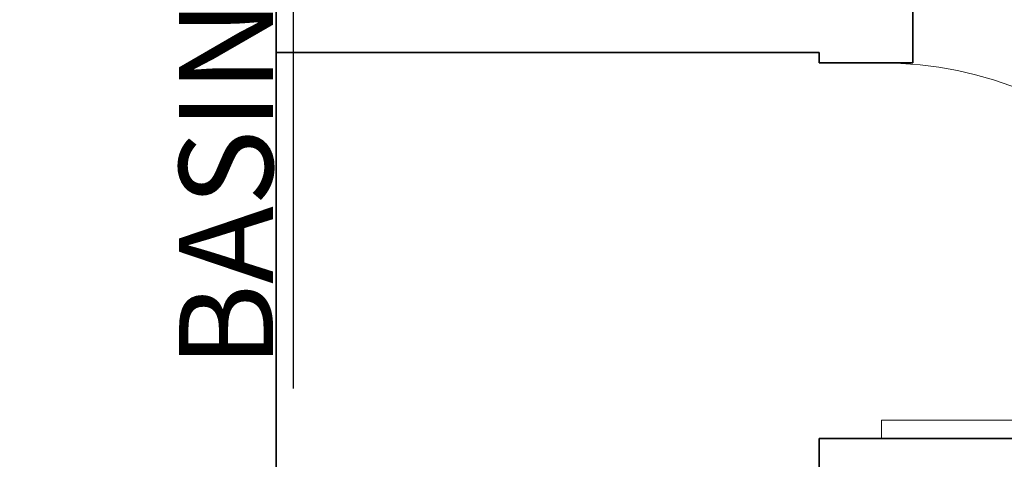
# Model space of a CAD drawing. Units: inches. Extents: x 3321 to 5237, y 11 to 1752.
# Tile 38 of 43: x 4916 to 5010, y 1556 to 1598. Entities that reach past the tile are written whole.
import ezdxf

# ---------------------------------------------------------------- set-up
doc = ezdxf.new("R2010")
doc.units = ezdxf.units.IN
for name, color, linetype, lineweight in [('A-ANNO-DIMS', 2, 'Continuous', 18), ('A-DOOR', 4, 'Continuous', 18), ('A-WALL', 7, 'Continuous', 35)]:
    doc.layers.add(name, color=color, linetype=linetype, lineweight=lineweight)
doc.styles.get("Standard").update_dxf_attribs({"font": 'arial.ttf'})
doc.dimstyles.new('ISO-25', dxfattribs={"dimtxt": 9, "dimasz": 2.5, "dimexe": 1.25, "dimexo": 0.625, "dimtad": 1, "dimdec": 1, "dimlunit": 3, "dimtxsty": 'Standard', "dimcen": 2.5, "dimclrd": 4, "dimclre": 4, "dimclrt": 256, "dimadec": 0, "dimazin": 0, "dimtfac": 1, "dimtdec": 1, "dimtmove": 0, "dimatfit": 3, "dimfxl": 1, "dimarcsym": 0})

# ---------------------------------------------------------------- blocks, each defined once
blk = doc.blocks.new('*U4')
for p, q in [((0, 0), (0, -6)), ((-36, 0), (-36, -6))]:
    blk.add_line(p, q)
blk.add_lwpolyline([(0, 0), (0, 36), (-1.75, 36), (-1.75, 0)], close=True)
blk.add_arc((0, 0), 36, 90, 180)
blk = doc.blocks.new('*D201')
at = {"layer": 'A-ANNO-DIMS', "color": 4, "lineweight": -2, "transparency": 16777216}
for p, q in [((4943.459, 1678.339), (4940.467, 1678.339)), ((4941.717, 1675.839), (4941.717, 1665.058)), ((4943.459, 1662.558), (4940.467, 1662.558)), ((4941.717, 1662.558), (4941.717, 1563.124))]:
    blk.add_line(p, q, dxfattribs=at)
at = {"layer": 'A-ANNO-DIMS', "color": 4, "transparency": 16777216}
for points in [[(4941.3, 1675.839), (4942.134, 1675.839), (4941.717, 1678.339)], [(4941.3, 1665.058), (4942.134, 1665.058), (4941.717, 1662.558)]]:
    blk.add_solid(points, dxfattribs=at)
at = {"layer": 'Defpoints', "color": 0, "transparency": 16777216}
for p in [(4944.084, 1678.339), (4941.717, 1662.558), (4944.084, 1662.558)]:
    blk.add_point(p, dxfattribs=at)
at = {"layer": 'A-ANNO-DIMS', "transparency": 16777216, "insert": (4936.439, 1611.591), "char_height": 9, "attachment_point": 5, "rotation": 90}
blk.add_mtext('BASIN 1\'-4" TYP.', dxfattribs=at)

msp = doc.modelspace()

# ---------------------------------------------------------------- linework, layer by layer
at = {"layer": 'A-WALL'}
for p, q in [((4940.084, 1687.339), (4940.084, 1425.339)), ((5001.084, 1644.339), (5001.084, 1594.339)), ((4992.084, 1595.339), (4940.084, 1595.339)), ((4992.084, 1595.339), (4992.084, 1594.339)), ((5001.084, 1594.339), (4992.084, 1594.339)), ((4992.084, 1558.339), (4992.084, 1479.339)), ((5121.084, 1558.339), (4992.084, 1558.339))]:
    msp.add_line(p, q, dxfattribs=at)

# ---------------------------------------------------------------- block references
at = {"layer": 'A-DOOR', "rotation": 270}
msp.add_blockref('*U4', (4998.084, 1558.339), dxfattribs=at)

# ---------------------------------------------------------------- dimensions: what is measured, and where the dimension line sits
at = {"layer": 'A-ANNO-DIMS'}
dim = msp.add_linear_dim(base=(4941.717, 1662.558), p1=(4944.084, 1678.339), p2=(4944.084, 1662.558), angle=270, text='BASIN <> TYP.', dimstyle='ISO-25', override={"dimdec": 1, "dimlfac": 1, "dimrnd": 0, "dimzin": 1, "dimdsep": 46, "dimlunit": 4, "dimfrac": 2}, dxfattribs=at)
dim.commit()
dim.dimension.update_dxf_attribs({"geometry": '*D201', "text_midpoint": (4936.439, 1611.591)})

doc.saveas('drawing.dxf')
